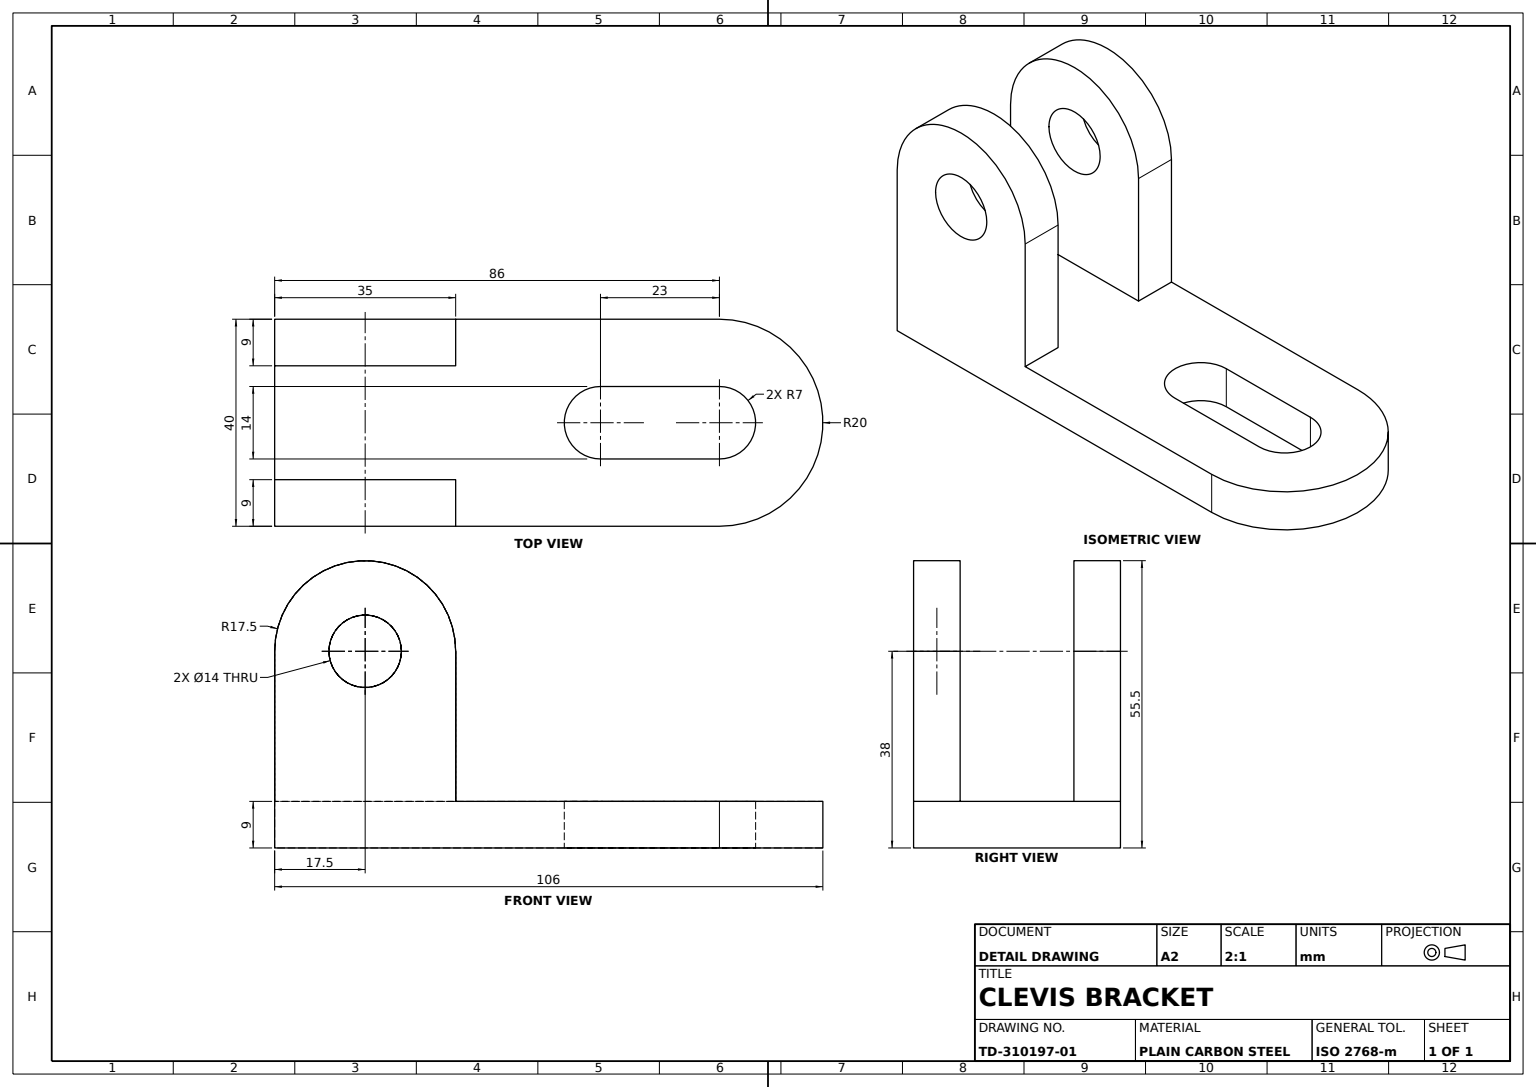
from build123d import *

# Parameters (mm, degrees)
SLOTTED_BASE_PLATE_DEPTH    = 9
CLEVIS_EAR_PROFILE_SKETCH_R = 7
CLEVIS_EAR_1_DEPTH          = 9
CLEVIS_START                = -31
SKETCH3_3_R                 = 7
CLEVIS_EAR_2_DEPTH          = 9


with BuildPart() as part:
    # Base Plate Slot Profile Sketch → Slotted Base Plate (new body)
    with BuildSketch(Plane(origin=(0, 0, 0), x_dir=(1, 0, 0), z_dir=(0, 1, 0))):
        with BuildLine():
            Line((0, 20), (0, -20))
            Line((0, -20), (86, -20))
            ThreePointArc((86, -20), (106, 0), (86, 20))
            Line((86, 20), (0, 20))
        make_face()
        with BuildLine():
            Line((86, -7), (63, -7))
            ThreePointArc((63, -7), (56, 0), (63, 7))
            Line((63, 7), (86, 7))
            ThreePointArc((86, 7), (93, 0), (86, -7))
        make_face(mode=Mode.SUBTRACT)
    extrude(amount=SLOTTED_BASE_PLATE_DEPTH)

    # Clevis Ear Profile Sketch → Clevis Ear 1 (add)
    with BuildSketch(Plane.XY.offset(20)):
        with BuildLine():
            Line((0, 38), (0, 9))
            Line((0, 9), (35, 9))
            Line((35, 9), (35, 38))
            ThreePointArc((35, 38), (17.5, 55.5), (0, 38))
        make_face()
        with Locations((17.5, 38)):
            Circle(CLEVIS_EAR_PROFILE_SKETCH_R, mode=Mode.SUBTRACT)
    extrude(amount=-CLEVIS_EAR_1_DEPTH)

    # Sketch3_3 → Clevis Ear 2 (add)
    with BuildSketch(Plane.XY.offset(20).offset(CLEVIS_START)):
        with BuildLine():
            Line((0, 38), (0, 9))
            Line((0, 9), (0, 0))
            Line((0, 0), (86, 0))
            Line((86, 0), (86, 9))
            Line((86, 9), (35, 9))
            Line((35, 9), (35, 38))
            ThreePointArc((35, 38), (17.5, 55.5), (0, 38))
        make_face()
        with Locations((17.5, 38)):
            Circle(SKETCH3_3_R, mode=Mode.SUBTRACT)
    extrude(amount=-CLEVIS_EAR_2_DEPTH)


solid = part.part
